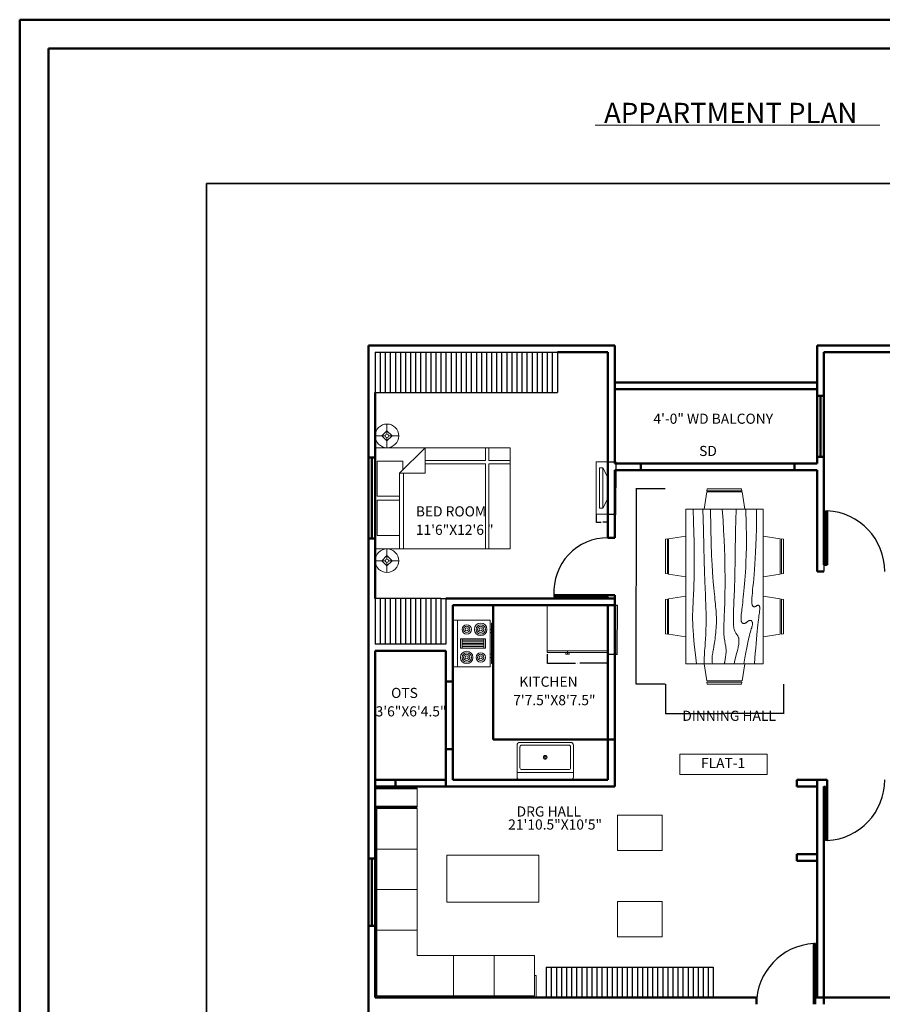
# Model space of a CAD drawing. Units: inches. Extents: x 1493 to 2377, y 814 to 2191.
# Tile 3 of 4: x 1493 to 2004, y 1607 to 2191. Entities that reach past the tile are written whole.
import ezdxf

# ---------------------------------------------------------------- set-up
doc = ezdxf.new("R2010")
doc.units = ezdxf.units.IN
for name, color, linetype, lineweight in [('A-ANNO-DIMS', 2, 'Continuous', 18), ('A-ANNO-SYMB', 2, 'Continuous', 18), ('A-ANNO-TEXT', 3, 'Continuous', 18), ('A-ANNO-TTLB', 7, 'Continuous', 35), ('A-AREA-IDEN', 7, 'Continuous', 18), ('A-DOOR', 4, 'Continuous', 25), ('A-EQPM', 9, 'Continuous', 18), ('A-FLOR-FIXT', 8, 'Continuous', 18), ('A-FURN', 8, 'Continuous', 18), ('A-GLAZ', 4, 'Continuous', 25), ('A-WALL', 7, 'Continuous', 50)]:
    doc.layers.add(name, color=color, linetype=linetype, lineweight=lineweight)
doc.styles.get("Standard").update_dxf_attribs({"font": 'arial.ttf'})
doc.dimstyles.get("Standard").update_dxf_attribs({"dimtxt": 0.18, "dimasz": 0.18, "dimexe": 0.18, "dimexo": 0.0625, "dimgap": 0.09, "dimtad": 0, "dimtih": 1, "dimtoh": 1, "dimdec": 4, "dimzin": 0, "dimdsep": 46, "dimtxsty": 'Standard', "dimcen": 0.09, "dimadec": 0, "dimazin": 0, "dimtfac": 1, "dimtdec": 4, "dimtofl": 0, "dimtmove": 0, "dimatfit": 3, "dimfxl": 1, "dimtolj": 1, "dimtzin": 0, "dimarcsym": 0})

# ---------------------------------------------------------------- blocks, each defined once
blk = doc.blocks.new('Lamp - Table')
for p, q in [((0, 7), (0, 1)), ((-1, 0), (-7, 0)), ((0, 3), (-3, 0)), ((-3, 0), (0, -3)), ((3, 0), (0, 3)), ((0, -3), (3, 0)), ((1, 0), (7, 0)), ((0, -1), (0, -7))]:
    blk.add_line(p, q)
for radius in [7, 1]:
    blk.add_circle((0, 0), radius)
blk = doc.blocks.new('Range-Oven - 30 in top')
for p, q in [((0, -3), (30, -3)), ((12, -6), (18, -6)), ((13, -20), (13, -6)), ((14, -6), (14, -20)), ((15, -20), (15, -6)), ((16, -6), (16, -20)), ((17, -20), (17, -6)), ((6, -24), (6, -25)), ((8, -25), (8, -24)), ((18, -20), (12, -20)), ((22, -25), (22, -24)), ((24, -24), (24, -25))]:
    blk.add_line(p, q)
for points in [[(0, -24), (0, 0), (30, 0), (30, -24)], [(12, -21), (12, -5), (18, -5), (18, -21)], [(2, -26), (2, -25), (28, -25), (28, -26)]]:
    blk.add_lwpolyline(points, close=True)
for centre, radius in [((6, -9), 4), ((6, -9), 3), ((24, -9), 3), ((6, -9), 2), ((6, -9), 1), ((24, -9), 2), ((24, -9), 1), ((6, -18), 3), ((6, -18), 2), ((6, -18), 1), ((24, -18), 4), ((24, -18), 3), ((24, -18), 2), ((24, -18), 1)]:
    blk.add_circle(centre, radius)
blk = doc.blocks.new('Refrigerator-2 door - 36 in top')
for p, q in [((0, -26.999999), (36, -26.999999)), ((11, -27.999999), (11, -28.999999)), ((11, -28.999999), (13, -28.999999)), ((12, -26.999999), (12, -28.999999)), ((13, -28.999999), (13, -27.999999))]:
    blk.add_line(p, q)
blk.add_lwpolyline([(0, -27.999999), (0, 0), (36, 0), (36, -27.999999)], close=True)
blk = doc.blocks.new('Bed - Queen')
for p, q in [((0, -80), (0, 0)), ((0, 0), (60, 0)), ((60, 0), (60, -80)), ((8, -1.2), (28.8, -1.2)), ((8, -14.4), (8, -1.2)), ((28.8, -1.2), (28.8, -14.4)), ((31.2, -1.2), (52, -1.2)), ((31.2, -14.4), (31.2, -1.2)), ((52, -1.2), (52, -16.4)), ((0, -14.4), (44.8, -14.4)), ((44.8, -16.8), (0, -16.8)), ((60, -29.6), (44.8, -14.4)), ((44.8, -14.4), (44.8, -29.6)), ((52, -16.4), (46.8, -16.4)), ((44.8, -29.6), (60, -29.6)), ((50.4, -29.6), (50.4, -65.35)), ((52.4, -29.6), (52.4, -65.35)), ((50.4, -65.35), (0, -65.35)), ((50.4, -67.35), (0, -67.35)), ((50.4, -67.35), (50.4, -80)), ((60, -65.35), (52.4, -65.35)), ((60, -67.35), (52.4, -67.35)), ((52.4, -67.35), (52.4, -80)), ((60, -80), (0, -80))]:
    blk.add_line(p, q)
blk = doc.blocks.new('Sink-single - 30 in top')
blk.add_line((-15, -3.999996), (15, -3.999996))
for points in [[(-13.5, 0), (13.5, 0)], [(-15, -18.499996), (-15, -1.5)], [(15, -1.5), (15, -18.499996)], [(-13.5, -17.499996), (-13.5, -6.499996)], [(-12.5, -5.499996), (12.5, -5.499996)], [(13.5, -6.499996), (13.5, -17.499996)], [(13.5, -19.999996), (-13.5, -19.999996)], [(12.5, -18.499996), (-12.5, -18.499996)]]:
    blk.add_lwpolyline(points)
for radius in [1, 0.5]:
    blk.add_circle((0, -11.999996), radius)
for centre, radius, start, end in [((-13.5, -1.5), 1.5, 90, 180), ((13.5, -1.5), 1.5, 0, 90), ((-12.5, -6.499996), 1, 90, 180), ((12.5, -6.499996), 1, 0, 90), ((-13.5, -18.499996), 1.5, 180, 270), ((-12.5, -17.499996), 1, 180, 270), ((12.5, -17.499996), 1, 270, 0), ((13.5, -18.499996), 1.5, 270, 0)]:
    blk.add_arc(centre, radius, start, end)
blk = doc.blocks.new('Dining Set - 36 x 72 in.')
for p, q in [((-22, 27.5), (-22.1562, 26.50042)), ((-22, 27.5), (-6, 27.5)), ((-5.8437, 26.49966), (-6, 27.5)), ((6, 27.5), (5.8438, 26.50042)), ((6, 27.5), (22, 27.5)), ((22.1563, 26.49966), (22, 27.5)), ((-22.2343, 26.00059), (-23.4847, 17.99762)), ((-22.2304, 26), (-5.7608, 26)), ((-5.8416, 26.5), (-22.1534, 26.5)), ((-4.5152, 17.99762), (-5.7655, 25.99926)), ((5.7657, 26.00059), (4.5153, 17.99762)), ((5.7696, 26), (22.2392, 26)), ((22.1584, 26.5), (5.8466, 26.5)), ((23.4848, 17.99762), (22.2345, 25.99926)), ((36, 18), (-36, 18)), ((-36, 18), (-36, -18)), ((36, -18), (36, 18)), ((-44.0006, 8.23428), (-35.9976, 9.48474)), ((44.0006, 8.23428), (35.9976, 9.48474)), ((-45.5, 8), (-44.5004, 8.15617)), ((-45.5, 8), (-45.5, -8)), ((-44.5, -8.15843), (-44.5, 8.15338)), ((-44, 8.23041), (-44, -8.23915)), ((44, 8.23041), (44, -8.23915)), ((44.5, -8.15843), (44.5, 8.15338)), ((45.5, 8), (44.5005, 8.15617)), ((45.5, 8), (45.5, -8)), ((-44.4997, -8.15631), (-45.5, -8)), ((-35.9976, -9.48476), (-43.9993, -8.2345)), ((35.9976, -9.48476), (43.9993, -8.2345)), ((44.4997, -8.15631), (45.5, -8)), ((-36, -18), (36, -18)), ((-22.2343, -26.0006), (-23.4847, -17.99762)), ((-4.5152, -17.99762), (-5.7655, -25.99928)), ((5.7657, -26.0006), (4.5153, -17.99762)), ((23.4848, -17.99762), (22.2345, -25.99928)), ((-22.2304, -26), (-5.7608, -26)), ((-22, -27.5), (-22.1562, -26.50044)), ((-5.8416, -26.5), (-22.1534, -26.5)), ((-5.8437, -26.49967), (-6, -27.5)), ((5.7696, -26), (22.2392, -26)), ((6, -27.5), (5.8438, -26.50044)), ((22.1584, -26.5), (5.8466, -26.5)), ((22.1563, -26.49967), (22, -27.5)), ((-22, -27.5), (-6, -27.5)), ((6, -27.5), (22, -27.5))]:
    blk.add_line(p, q)
for points in [[(-36, 15), (-31.1772, 14.97754), (-26.8079, 14.91406), (-22.8538, 14.81543), (-19.276, 14.6875), (-16.0362, 14.53613), (-13.0957, 14.36718), (-10.4159, 14.18652), (-7.9583, 14), (-5.6904, 13.81315), (-3.6035, 13.63021), (-1.6954, 13.45508), (0.0365, 13.29166), (1.5945, 13.14388), (2.9811, 13.01562), (4.1988, 12.9108), (5.25, 12.83333), (6.1393, 12.78613), (6.8802, 12.76823), (7.4883, 12.77767), (7.9792, 12.8125), (8.3685, 12.87077), (8.6719, 12.95052), (8.9049, 13.0498), (9.0833, 13.16666), (9.2205, 13.29899), (9.3216, 13.44401), (9.3895, 13.59879), (9.4271, 13.76041), (9.4373, 13.92594), (9.4232, 14.09245), (9.3875, 14.257), (9.3333, 14.41666), (9.2638, 14.56917), (9.1836, 14.71484), (9.0975, 14.85465), (9.0104, 14.98958), (8.9272, 15.1206), (8.8529, 15.2487), (8.7922, 15.37483), (8.75, 15.5), (8.7305, 15.62467), (8.7344, 15.74739), (8.7617, 15.86621), (8.8125, 15.97916), (8.8867, 16.08431), (8.9844, 16.17968), (9.1055, 16.26334), (9.25, 16.33333), (9.4189, 16.38802), (9.6172, 16.42708), (9.8506, 16.45052), (10.125, 16.45833), (10.4463, 16.45052), (10.8203, 16.42708), (11.2529, 16.38802), (11.75, 16.33333), (12.3184, 16.26318), (12.9694, 16.17838), (13.7151, 16.07991), (14.5677, 15.96875), (15.5395, 15.84586), (16.6426, 15.71224), (17.8893, 15.56884), (19.2917, 15.41666), (20.859, 15.25667), (22.5879, 15.08984), (24.4721, 14.91715), (26.5052, 14.73958), (28.6809, 14.5581), (30.9929, 14.3737), (33.4347, 14.18733), (36, 14)], [(-36, 10), (-28.9766, 10.14274), (-23.1725, 10.20442), (-18.4241, 10.19775), (-14.5677, 10.13541), (-11.4399, 10.03011), (-8.877, 9.89453), (-6.7154, 9.74137), (-4.7917, 9.58333), (-2.9698, 9.43082), (-1.2246, 9.28515), (0.4415, 9.14534), (2.026, 9.01041), (3.5266, 8.87939), (4.9408, 8.7513), (6.266, 8.62516), (7.5, 8.5), (8.6411, 8.37549), (9.6914, 8.2539), (10.6538, 8.13818), (11.5312, 8.03125), (12.3267, 7.93603), (13.043, 7.85547), (13.6831, 7.79248), (14.25, 7.75), (14.7471, 7.7303), (15.1797, 7.73307), (15.5537, 7.75732), (15.875, 7.80208), (16.1494, 7.86637), (16.3828, 7.94922), (16.5811, 8.04964), (16.75, 8.16666), (16.8944, 8.29915), (17.0143, 8.44531), (17.1089, 8.60319), (17.1771, 8.77083), (17.218, 8.94629), (17.2305, 9.1276), (17.2137, 9.31282), (17.1667, 9.5), (17.0895, 9.6875), (16.987, 9.875), (16.8649, 10.0625), (16.7292, 10.25), (16.5856, 10.4375), (16.4401, 10.625), (16.2985, 10.8125), (16.1667, 11), (16.05, 11.18733), (15.9518, 11.3737), (15.8752, 11.5581), (15.8229, 11.73958), (15.798, 11.91715), (15.8034, 12.08984), (15.842, 12.25667), (15.9167, 12.41666), (16.0295, 12.56836), (16.1784, 12.70833), (16.3605, 12.83268), (16.5729, 12.9375), (16.8127, 13.01888), (17.0768, 13.07291), (17.3625, 13.0957), (17.6667, 13.08333), (17.9894, 13.03312), (18.3418, 12.94726), (18.7382, 12.82918), (19.1927, 12.68229), (19.7195, 12.51001), (20.3327, 12.31575), (21.0465, 12.10294), (21.875, 11.875), (22.8357, 11.63354), (23.959, 11.37304), (25.2786, 11.08618), (26.8282, 10.76562), (28.6414, 10.40405), (30.752, 9.99414), (33.1936, 9.52856), (36, 9)], [(-36, 5.5), (-30.7157, 5.3348), (-26.069, 5.20963), (-21.9946, 5.11767), (-18.4271, 5.05208), (-15.3009, 5.00602), (-12.5508, 4.97265), (-10.1112, 4.94515), (-7.9167, 4.91666), (-5.909, 4.88167), (-4.0586, 4.83984), (-2.3429, 4.79215), (-0.7396, 4.73958), (0.7739, 4.6831), (2.22, 4.6237), (3.6213, 4.56233), (5, 4.5), (6.373, 4.43782), (7.7344, 4.3776), (9.0723, 4.32129), (10.375, 4.27083), (11.6309, 4.22819), (12.8281, 4.19531), (13.9551, 4.17415), (15, 4.16666), (15.954, 4.17448), (16.819, 4.19791), (17.6001, 4.23698), (18.3021, 4.29166), (18.9299, 4.36198), (19.4883, 4.44791), (19.9823, 4.54948), (20.4167, 4.66666), (20.7969, 4.79899), (21.1302, 4.94401), (21.4245, 5.09879), (21.6875, 5.26041), (21.9271, 5.42594), (22.1511, 5.59245), (22.3672, 5.757), (22.5834, 5.91666), (22.8065, 6.06868), (23.0404, 6.21093), (23.2879, 6.34147), (23.5521, 6.45833), (23.8358, 6.55957), (24.142, 6.64323), (24.4735, 6.70735), (24.8334, 6.75), (25.2235, 6.76969), (25.642, 6.76692), (26.0858, 6.74267), (26.5521, 6.69791), (27.0379, 6.63362), (27.5404, 6.55078), (28.0565, 6.45036), (28.5834, 6.33333), (29.1242, 6.19987), (29.7071, 6.04687), (30.3661, 5.87044), (31.1354, 5.66666), (32.0493, 5.43164), (33.142, 5.16146), (34.4475, 4.85221), (36, 4.5)], [(-36, -1), (-30.7915, -0.6591), (-26.0195, -0.38216), (-21.6519, -0.16284), (-17.6563, 0.00521), (-14.0005, 0.12833), (-10.6523, 0.21289), (-7.5796, 0.26522), (-4.75, 0.29166), (-2.134, 0.29793), (0.2878, 0.28711), (2.5317, 0.26163), (4.6146, 0.22396), (6.5529, 0.17651), (8.3633, 0.12174), (10.0623, 0.06209), (11.6667, 0), (13.1899, -0.06201), (14.6341, -0.1211), (15.9982, -0.17432), (17.2813, -0.21875), (18.4823, -0.25147), (19.6003, -0.26953), (20.6343, -0.27002), (21.5834, -0.25), (22.4481, -0.20768), (23.2357, -0.14584), (23.9549, -0.06836), (24.6146, 0.02083), (25.2235, 0.11784), (25.7904, 0.21875), (26.3241, 0.31966), (26.8334, 0.41666), (27.3265, 0.50618), (27.8099, 0.58593), (28.2894, 0.65397), (28.7709, 0.70833), (29.2601, 0.74707), (29.763, 0.76823), (30.2855, 0.76985), (30.8334, 0.75), (31.4088, 0.70784), (31.9994, 0.64713), (32.589, 0.57275), (33.1615, 0.48958), (33.7008, 0.4025), (34.1908, 0.3164), (34.6153, 0.23616), (34.9584, 0.16666), (35.2099, 0.11165), (35.3848, 0.07031), (35.504, 0.04069), (35.5886, 0.02083), (35.6594, 0.00879), (35.7377, 0.0026), (35.8442, 0.00032), (36, 0)], [(-36, -6.5), (-27.1843, -6.31267), (-20.084, -6.1263), (-14.469, -5.9419), (-10.1094, -5.76042), (-6.7752, -5.58285), (-4.2363, -5.41016), (-2.2629, -5.24333), (-0.625, -5.08334), (0.8708, -4.93099), (2.2715, -4.78646), (3.5872, -4.64974), (4.8281, -4.52084), (6.0046, -4.39974), (7.127, -4.28646), (8.2053, -4.18099), (9.25, -4.08334), (10.2705, -3.99382), (11.2734, -3.91407), (12.2647, -3.84603), (13.25, -3.79167), (14.2354, -3.75293), (15.2266, -3.73177), (16.2295, -3.73015), (17.25, -3.75), (18.2912, -3.79248), (19.3451, -3.85547), (20.4009, -3.93604), (21.4479, -4.03125), (22.4754, -4.13819), (23.4727, -4.25391), (24.4289, -4.37549), (25.3334, -4.5), (26.1785, -4.62492), (26.9694, -4.74935), (27.7145, -4.87281), (28.4219, -4.99479), (29.1, -5.11483), (29.7572, -5.23242), (30.4016, -5.34709), (31.0417, -5.45834), (31.6837, -5.56437), (32.3262, -5.65821), (32.9658, -5.73153), (33.599, -5.77604), (34.2224, -5.78345), (34.8327, -5.74545), (35.4264, -5.65373), (36, -5.5)], [(-36, -10), (-26.4022, -9.81299), (-18.4675, -9.62891), (-11.9839, -9.45069), (-6.7396, -9.28125), (-2.5226, -9.12354), (0.8789, -8.98047), (3.6769, -8.85498), (6.0833, -8.75), (8.2767, -8.66765), (10.3021, -8.60677), (12.1712, -8.56543), (13.8958, -8.54167), (15.4876, -8.53353), (16.9583, -8.53907), (18.3197, -8.55632), (19.5834, -8.58334), (20.7616, -8.61841), (21.8685, -8.66081), (22.9188, -8.71004), (23.9271, -8.76563), (24.9081, -8.82707), (25.8763, -8.89388), (26.8465, -8.96558), (27.8334, -9.04167), (28.8474, -9.12118), (29.8828, -9.20117), (30.93, -9.27824), (31.9792, -9.34896), (33.0205, -9.40991), (34.0443, -9.45768), (35.0407, -9.48885), (36, -9.5)], [(-36, -14.5), (-30.0881, -14.33513), (-25.0332, -14.21224), (-20.7312, -14.12647), (-17.0781, -14.07292), (-13.97, -14.04671), (-11.3027, -14.04297), (-8.9724, -14.05681), (-6.875, -14.08334), (-4.9224, -14.11833), (-3.0905, -14.16016), (-1.3709, -14.20785), (0.2448, -14.26042), (1.7647, -14.3169), (3.1973, -14.3763), (4.5507, -14.43767), (5.8333, -14.5), (7.0554, -14.5621), (8.235, -14.62175), (9.3922, -14.67652), (10.5469, -14.72396), (11.7192, -14.76164), (12.929, -14.78711), (14.1965, -14.79794), (15.5417, -14.79167), (16.9933, -14.76424), (18.6152, -14.70508), (20.4804, -14.60197), (22.6615, -14.44271), (25.2312, -14.21509), (28.2624, -13.9069), (31.8277, -13.50594), (36, -13)]]:
    blk.add_lwpolyline(points)
blk = doc.blocks.new('AC-SPLIT-UNIT')
for p, q in [((-2, 27.5), (-2, -3.65)), ((-2, 27.5), (5, 27.5)), ((0, 24), (2, 24)), ((0, 24), (0, 0)), ((2, 24), (2, 0)), ((2, 24), (5, 18.22)), ((2, 0), (5, 5.78)), ((-2, -3.65), (5, -3.65)), ((0, 0), (2, 0))]:
    blk.add_line(p, q)
blk = doc.blocks.new('*D24')
at = {"layer": 'A-ANNO-DIMS', "color": 0, "lineweight": -2, "transparency": 16777216}
for p, q in [((1841.9, 1928.89), (1846.69, 1928.89)), ((1846.51, 1928.71), (1846.51, 1913.5)), ((1846.51, 1897.92), (1846.51, 1913.13)), ((1841.9, 1897.74), (1846.69, 1897.74))]:
    blk.add_line(p, q, dxfattribs=at)
at = {"layer": 'A-ANNO-DIMS', "color": 0, "transparency": 16777216}
for points in [[(1846.48, 1928.71), (1846.54, 1928.71), (1846.51, 1928.89)], [(1846.48, 1897.92), (1846.54, 1897.92), (1846.51, 1897.74)]]:
    blk.add_solid(points, dxfattribs=at)
at = {"layer": 'Defpoints', "color": 0, "transparency": 16777216}
for p in [(1841.83, 1928.89), (1846.51, 1928.89), (1841.83, 1897.74)]:
    blk.add_point(p, dxfattribs=at)
at = {"layer": 'A-ANNO-DIMS', "color": 0, "transparency": 16777216, "insert": (1846.51, 1913.32), "char_height": 0.18, "attachment_point": 5}
blk.add_mtext('\\A1;AC SPLIT UNIT 31 TYP.', dxfattribs=at)
blk = doc.blocks.new('*D25')
at = {"layer": 'A-ANNO-DIMS', "color": 0, "lineweight": -2, "transparency": 16777216}
for p, q in [((1834.83, 1897.68), (1834.83, 1892.89)), ((1841.83, 1897.68), (1841.83, 1892.89)), ((1835.01, 1893.07), (1837.88, 1893.07)), ((1841.65, 1893.07), (1838.79, 1893.07))]:
    blk.add_line(p, q, dxfattribs=at)
at = {"layer": 'A-ANNO-DIMS', "color": 0, "transparency": 16777216}
for points in [[(1835.01, 1893.1), (1835.01, 1893.04), (1834.83, 1893.07)], [(1841.65, 1893.1), (1841.65, 1893.04), (1841.83, 1893.07)]]:
    blk.add_solid(points, dxfattribs=at)
at = {"layer": 'Defpoints', "color": 0, "transparency": 16777216}
for p in [(1834.83, 1897.74), (1841.83, 1897.74), (1841.83, 1893.07)]:
    blk.add_point(p, dxfattribs=at)
at = {"layer": 'A-ANNO-DIMS', "color": 0, "transparency": 16777216, "insert": (1838.33, 1893.07), "char_height": 0.18, "attachment_point": 5}
blk.add_mtext('\\A1;7 TYP.', dxfattribs=at)
blk = doc.blocks.new('*D30')
at = {"layer": 'A-ANNO-DIMS', "color": 0, "lineweight": -2, "transparency": 16777216}
for p, q in [((1875.78, 1912.92), (1858.28, 1912.92)), ((1858.46, 1912.74), (1858.46, 1855.18)), ((1858.46, 1797.25), (1858.46, 1854.81)), ((1875.78, 1797.07), (1858.28, 1797.07))]:
    blk.add_line(p, q, dxfattribs=at)
at = {"layer": 'A-ANNO-DIMS', "color": 0, "transparency": 16777216}
for points in [[(1858.43, 1912.74), (1858.49, 1912.74), (1858.46, 1912.92)], [(1858.43, 1797.25), (1858.49, 1797.25), (1858.46, 1797.07)]]:
    blk.add_solid(points, dxfattribs=at)
at = {"layer": 'Defpoints', "color": 0, "transparency": 16777216}
for p in [(1875.84, 1912.92), (1858.46, 1797.07), (1875.84, 1797.07)]:
    blk.add_point(p, dxfattribs=at)
at = {"layer": 'A-ANNO-DIMS', "color": 0, "transparency": 16777216, "insert": (1858.46, 1854.99), "char_height": 0.18, "attachment_point": 5}
blk.add_mtext('\\A1;DINING SET 116', dxfattribs=at)
blk = doc.blocks.new('*D31')
at = {"layer": 'A-ANNO-DIMS', "color": 0, "lineweight": -2, "transparency": 16777216}
for p, q in [((1875.84, 1797), (1875.84, 1779.51)), ((1945.87, 1797), (1945.87, 1779.51)), ((1876.02, 1779.69), (1910.64, 1779.69)), ((1945.69, 1779.69), (1911.07, 1779.69))]:
    blk.add_line(p, q, dxfattribs=at)
at = {"layer": 'A-ANNO-DIMS', "color": 0, "transparency": 16777216}
for points in [[(1876.02, 1779.72), (1876.02, 1779.66), (1875.84, 1779.69)], [(1945.69, 1779.72), (1945.69, 1779.66), (1945.87, 1779.69)]]:
    blk.add_solid(points, dxfattribs=at)
at = {"layer": 'Defpoints', "color": 0, "transparency": 16777216}
for p in [(1875.84, 1797.07), (1945.87, 1797.07), (1945.87, 1779.69)]:
    blk.add_point(p, dxfattribs=at)
at = {"layer": 'A-ANNO-DIMS', "color": 0, "transparency": 16777216, "insert": (1910.85, 1779.69), "char_height": 0.18, "attachment_point": 5}
blk.add_mtext('\\A1;70', dxfattribs=at)
blk = doc.blocks.new('*D34')
at = {"layer": 'A-ANNO-DIMS', "color": 0, "lineweight": -2, "transparency": 16777216}
for p, q in [((1805.83, 1814.8), (1805.83, 1809.29)), ((1841.83, 1814.8), (1841.83, 1809.29)), ((1806.01, 1809.47), (1822.58, 1809.47)), ((1841.65, 1809.47), (1825.08, 1809.47))]:
    blk.add_line(p, q, dxfattribs=at)
at = {"layer": 'A-ANNO-DIMS', "color": 0, "transparency": 16777216}
for points in [[(1806.01, 1809.5), (1806.01, 1809.44), (1805.83, 1809.47)], [(1841.65, 1809.5), (1841.65, 1809.44), (1841.83, 1809.47)]]:
    blk.add_solid(points, dxfattribs=at)
at = {"layer": 'Defpoints', "color": 0, "transparency": 16777216}
for p in [(1805.83, 1814.87), (1841.83, 1814.87), (1841.83, 1809.47)]:
    blk.add_point(p, dxfattribs=at)
at = {"layer": 'A-ANNO-DIMS', "color": 0, "transparency": 16777216, "insert": (1823.83, 1809.47), "char_height": 0.18, "attachment_point": 5}
blk.add_mtext('\\A1;REFRIGERATOR 36', dxfattribs=at)
blk = doc.blocks.new('*D35')
at = {"layer": 'A-ANNO-DIMS', "color": 0, "lineweight": -2, "transparency": 16777216}
for p, q in [((1841.9, 1843.87), (1847.41, 1843.87)), ((1847.23, 1843.69), (1847.23, 1829.55)), ((1847.23, 1815.05), (1847.23, 1829.19)), ((1841.9, 1814.87), (1847.41, 1814.87))]:
    blk.add_line(p, q, dxfattribs=at)
at = {"layer": 'A-ANNO-DIMS', "color": 0, "transparency": 16777216}
for points in [[(1847.2, 1843.69), (1847.26, 1843.69), (1847.23, 1843.87)], [(1847.2, 1815.05), (1847.26, 1815.05), (1847.23, 1814.87)]]:
    blk.add_solid(points, dxfattribs=at)
at = {"layer": 'Defpoints', "color": 0, "transparency": 16777216}
for p in [(1841.83, 1843.87), (1847.23, 1843.87), (1841.83, 1814.87)]:
    blk.add_point(p, dxfattribs=at)
at = {"layer": 'A-ANNO-DIMS', "color": 0, "transparency": 16777216, "insert": (1847.23, 1829.37), "char_height": 0.18, "attachment_point": 5}
blk.add_mtext('\\A1;29', dxfattribs=at)

msp = doc.modelspace()

# ---------------------------------------------------------------- linework, layer by layer
at = {"layer": 'A-ANNO-SYMB'}
msp.add_lwpolyline([(1884.39, 1755.7), (1936.09, 1755.7), (1936.09, 1743.61), (1884.39, 1743.61)], close=True, dxfattribs=at)
at = {"layer": 'A-ANNO-TEXT'}
msp.add_line((1834.32, 2128.42), (2002.99, 2128.42), dxfattribs=at)
at = {"layer": 'A-ANNO-TTLB'}
for q in [(1603.83, 914.87), (2271.83, 2093.87)]:
    msp.add_line((1603.83, 2093.87), q, dxfattribs=at)
at = {"layer": 'A-DOOR'}
for p, q in [((1970.83, 1899.87), (1971.83, 1899.87)), ((1970.83, 1899.87), (1970.83, 1867.87)), ((1969.83, 1867.87), (1969.83, 1863.87)), ((1809.83, 1849.87), (1809.83, 1848.87)), ((1970.83, 1736.37), (1969.83, 1736.37)), ((1970.83, 1736.37), (1970.83, 1704.37)), ((1971.83, 1704.37), (1970.83, 1704.37)), ((1964.83, 1643.37), (1963.83, 1643.37)), ((1964.83, 1643.37), (1964.83, 1607.37))]:
    msp.add_line(p, q, dxfattribs=at)
for centre, radius, start, end in [((1969.77, 1863.87), 36.06, 0, 86.72685), ((1841.83, 1851.81), 32.06, 90, 183.47141), ((1969.77, 1740.37), 36.06, 273.27315, 360), ((1965.89, 1607.37), 36.06, 93.27315, 180)]:
    msp.add_arc(centre, radius, start, end, dxfattribs=at)
at = {"layer": 'A-FURN'}
for p, q in [((1728.83, 1724.37), (1728.83, 1735.37)), ((1704.83, 1723.37), (1704.83, 1612.37)), ((1728.83, 1723.37), (1704.83, 1723.37)), ((1709.83, 1724.37), (1709.83, 1723.37)), ((1728.83, 1723.37), (1728.83, 1636.37)), ((1728.83, 1699.37), (1704.83, 1699.37)), ((1728.83, 1675.37), (1704.83, 1675.37)), ((1728.83, 1651.37), (1704.83, 1651.37)), ((1798.36, 1636.37), (1728.83, 1636.37)), ((1750.36, 1636.37), (1750.36, 1612.37)), ((1774.36, 1636.37), (1774.36, 1612.37)), ((1798.36, 1636.37), (1798.36, 1612.37)), ((1799.36, 1624.37), (1798.36, 1624.37)), ((1799.36, 1624.37), (1799.36, 1611.37)), ((1798.36, 1612.37), (1704.83, 1612.37))]:
    msp.add_line(p, q, dxfattribs=at)
for points in [[(1847.43, 1719.55), (1873.89, 1719.55), (1873.89, 1698.59), (1847.43, 1698.59)], [(1746.4, 1695.69), (1800.95, 1695.69), (1800.95, 1667.95), (1746.4, 1667.95)], [(1847.43, 1668.28), (1873.89, 1668.28), (1873.89, 1647.31), (1847.43, 1647.31)]]:
    msp.add_lwpolyline(points, close=True, dxfattribs=at)
at = {"layer": 'A-GLAZ'}
for p, q in [((1703.83, 1993.87), (1808.83, 1993.87)), ((1703.83, 1993.87), (1703.83, 1969.87)), ((1706.83, 1993.87), (1706.83, 1969.87)), ((1709.83, 1993.87), (1709.83, 1969.87)), ((1712.83, 1993.87), (1712.83, 1969.87)), ((1715.83, 1993.87), (1715.83, 1969.87)), ((1718.83, 1993.87), (1718.83, 1969.87)), ((1721.83, 1993.87), (1721.83, 1969.87)), ((1724.83, 1993.87), (1724.83, 1969.87)), ((1727.83, 1993.87), (1727.83, 1969.87)), ((1730.83, 1993.87), (1730.83, 1969.87)), ((1733.83, 1993.87), (1733.83, 1969.87)), ((1736.83, 1993.87), (1736.83, 1969.87)), ((1739.83, 1993.87), (1739.83, 1969.87)), ((1742.83, 1993.87), (1742.83, 1969.87)), ((1745.83, 1993.87), (1745.83, 1969.87)), ((1748.83, 1993.87), (1748.83, 1969.87)), ((1751.83, 1993.87), (1751.83, 1969.87)), ((1754.83, 1993.87), (1754.83, 1969.87)), ((1757.83, 1993.87), (1757.83, 1969.87)), ((1760.83, 1993.87), (1760.83, 1969.87)), ((1763.83, 1993.87), (1763.83, 1969.87)), ((1766.83, 1993.87), (1766.83, 1969.87)), ((1769.83, 1993.87), (1769.83, 1969.87)), ((1772.83, 1993.87), (1772.83, 1969.87)), ((1775.83, 1993.87), (1775.83, 1969.87)), ((1778.83, 1993.87), (1778.83, 1969.87)), ((1781.83, 1993.87), (1781.83, 1969.87)), ((1784.83, 1993.87), (1784.83, 1969.87)), ((1787.83, 1993.87), (1787.83, 1969.87)), ((1790.83, 1993.87), (1790.83, 1969.87)), ((1793.83, 1993.87), (1793.83, 1969.87)), ((1796.83, 1993.87), (1796.83, 1969.87)), ((1799.83, 1993.87), (1799.83, 1969.87)), ((1802.83, 1993.87), (1802.83, 1969.87)), ((1805.83, 1993.87), (1805.83, 1969.87)), ((1808.83, 1993.87), (1808.83, 1969.87)), ((1808.83, 1993.87), (1811.83, 1993.87)), ((1811.83, 1993.87), (1811.83, 1969.87)), ((1703.83, 1969.87), (1811.83, 1969.87)), ((1742.83, 1847.87), (1703.83, 1847.87)), ((1703.83, 1847.87), (1703.83, 1820.87)), ((1706.83, 1847.87), (1706.83, 1820.87)), ((1709.83, 1847.87), (1709.83, 1820.87)), ((1712.83, 1847.87), (1712.83, 1820.87)), ((1715.83, 1847.87), (1715.83, 1820.87)), ((1718.83, 1847.87), (1718.83, 1820.87)), ((1721.83, 1847.87), (1721.83, 1820.87)), ((1724.83, 1847.87), (1724.83, 1820.87)), ((1727.83, 1847.87), (1727.83, 1820.87)), ((1730.83, 1847.87), (1730.83, 1820.87)), ((1733.83, 1847.87), (1733.83, 1820.87)), ((1736.83, 1847.87), (1736.83, 1820.87)), ((1739.83, 1847.87), (1739.83, 1820.87)), ((1742.83, 1847.87), (1742.83, 1820.87)), ((1742.83, 1847.87), (1745.83, 1847.87)), ((1745.83, 1847.87), (1745.83, 1820.87)), ((1745.83, 1820.87), (1703.83, 1820.87)), ((1805.27, 1629.37), (1904.27, 1629.37)), ((1805.27, 1629.37), (1805.27, 1611.37)), ((1808.27, 1629.37), (1808.27, 1611.37)), ((1811.27, 1629.37), (1811.27, 1611.37)), ((1814.27, 1629.37), (1814.27, 1611.37)), ((1817.27, 1629.37), (1817.27, 1611.37)), ((1820.27, 1629.37), (1820.27, 1611.37)), ((1823.27, 1629.37), (1823.27, 1611.37)), ((1826.27, 1629.37), (1826.27, 1611.37)), ((1829.27, 1629.37), (1829.27, 1611.37)), ((1832.27, 1629.37), (1832.27, 1611.37)), ((1835.27, 1629.37), (1835.27, 1611.37)), ((1838.27, 1629.37), (1838.27, 1611.37)), ((1841.27, 1629.37), (1841.27, 1611.37)), ((1844.27, 1629.37), (1844.27, 1611.37)), ((1847.27, 1629.37), (1847.27, 1611.37)), ((1850.27, 1629.37), (1850.27, 1611.37)), ((1853.27, 1629.37), (1853.27, 1611.37)), ((1856.27, 1629.37), (1856.27, 1611.37)), ((1859.27, 1629.37), (1859.27, 1611.37)), ((1862.27, 1629.37), (1862.27, 1611.37)), ((1865.27, 1629.37), (1865.27, 1611.37)), ((1868.27, 1629.37), (1868.27, 1611.37)), ((1871.27, 1629.37), (1871.27, 1611.37)), ((1874.27, 1629.37), (1874.27, 1611.37)), ((1877.27, 1629.37), (1877.27, 1611.37)), ((1880.27, 1629.37), (1880.27, 1611.37)), ((1883.27, 1629.37), (1883.27, 1611.37)), ((1886.27, 1629.37), (1886.27, 1611.37)), ((1889.27, 1629.37), (1889.27, 1611.37)), ((1892.27, 1629.37), (1892.27, 1611.37)), ((1895.27, 1629.37), (1895.27, 1611.37)), ((1898.27, 1629.37), (1898.27, 1611.37)), ((1901.27, 1629.37), (1901.27, 1611.37)), ((1904.27, 1629.37), (1904.27, 1611.37))]:
    msp.add_line(p, q, dxfattribs=at)
at = {"layer": 'A-WALL'}
for p, q in [((1699.83, 1997.87), (1845.83, 1997.87)), ((1699.83, 1997.87), (1699.83, 1010.87)), ((1845.83, 1997.87), (1845.83, 1927.87)), ((1965.83, 1997.87), (1965.83, 1927.87)), ((1965.83, 1997.87), (2151.83, 1997.87)), ((1965.83, 1997.87), (1965.83, 1927.87)), ((1811.83, 1993.87), (1841.83, 1993.87)), ((1841.83, 1993.87), (1841.83, 1883.87)), ((1969.83, 1993.87), (1969.83, 1867.87)), ((1969.83, 1993.87), (1969.83, 1867.87)), ((1969.83, 1993.87), (2125.83, 1993.87)), ((1845.83, 1975.87), (1965.83, 1975.87)), ((1703.83, 1969.87), (1703.83, 1847.87)), ((1845.83, 1971.87), (1965.83, 1971.87)), ((1965.83, 1967.87), (1969.83, 1967.87)), ((1967.83, 1967.87), (1967.83, 1931.87)), ((1965.83, 1931.87), (1969.83, 1931.87)), ((1703.83, 1931.37), (1699.83, 1931.37)), ((1701.83, 1931.37), (1701.83, 1883.37)), ((1845.83, 1927.87), (1965.83, 1927.87)), ((1861.27, 1927.87), (1861.27, 1923.87)), ((1952.36, 1927.87), (1952.36, 1923.87)), ((1845.83, 1923.87), (1965.83, 1923.87)), ((1845.83, 1923.87), (1845.83, 1883.87)), ((1965.83, 1923.87), (1965.83, 1863.87)), ((1965.83, 1923.87), (1965.83, 1863.87)), ((1971.83, 1899.87), (1971.83, 1867.87)), ((1703.83, 1883.37), (1699.83, 1883.37)), ((1845.83, 1883.87), (1841.83, 1883.87)), ((1969.83, 1867.87), (1971.83, 1867.87)), ((1965.83, 1863.87), (1969.83, 1863.87)), ((1845.83, 1849.87), (1809.83, 1849.87)), ((1845.83, 1849.87), (1845.83, 1736.37)), ((1845.83, 1847.87), (1745.83, 1847.87)), ((1845.83, 1843.87), (1749.83, 1843.87)), ((1749.83, 1843.87), (1749.83, 1798.62)), ((1773.83, 1843.87), (1773.83, 1764.37)), ((1841.83, 1848.87), (1809.83, 1848.87)), ((1841.83, 1848.87), (1841.83, 1847.87)), ((1841.83, 1843.87), (1841.83, 1740.37)), ((1745.83, 1816.87), (1703.83, 1816.87)), ((1703.83, 1816.87), (1703.83, 1736.37)), ((1745.83, 1816.87), (1745.83, 1798.62)), ((1745.83, 1798.62), (1749.83, 1798.62)), ((1745.83, 1798.62), (1745.83, 1758.62)), ((1749.83, 1798.62), (1749.83, 1758.62)), ((1845.83, 1764.37), (1773.83, 1764.37)), ((1745.83, 1758.62), (1749.83, 1758.62)), ((1745.83, 1758.62), (1745.83, 1736.37)), ((1749.83, 1758.62), (1749.83, 1740.37)), ((1745.83, 1740.37), (1703.83, 1740.37)), ((1715.83, 1740.37), (1715.83, 1736.37)), ((1841.83, 1740.37), (1749.83, 1740.37)), ((1953.83, 1740.37), (1965.83, 1740.37)), ((1953.83, 1740.37), (1953.83, 1736.37)), ((1971.83, 1740.37), (1965.83, 1740.37)), ((1965.83, 1740.37), (1965.83, 1611.37)), ((1971.83, 1740.37), (1971.83, 1704.37)), ((1845.83, 1736.37), (1703.83, 1736.37)), ((1703.83, 1736.37), (1703.83, 1611.37)), ((1728.83, 1735.37), (1703.83, 1735.37)), ((1953.83, 1736.37), (1965.83, 1736.37)), ((1969.83, 1736.37), (1969.83, 1607.37)), ((1728.83, 1724.37), (1703.83, 1724.37)), ((1703.83, 1693.87), (1699.83, 1693.87)), ((1701.83, 1693.87), (1701.83, 1653.87)), ((1953.83, 1696.37), (1965.83, 1696.37)), ((1953.83, 1696.37), (1953.83, 1692.37)), ((1953.83, 1692.37), (1965.83, 1692.37)), ((1703.83, 1653.87), (1699.83, 1653.87)), ((1963.83, 1643.37), (1963.83, 1607.37)), ((1929.83, 1611.37), (1703.83, 1611.37)), ((1929.83, 1611.37), (1929.83, 1607.37)), ((2147.83, 1611.37), (1964.83, 1611.37))]:
    msp.add_line(p, q, dxfattribs=at)
for points in [[(1493.21, 2190.87), (2376.73, 2190.87), (2376.73, 813.94), (1493.21, 813.94)], [(1510.21, 2173.87), (2359.73, 2173.87), (2359.73, 830.94), (1510.21, 830.94)]]:
    msp.add_lwpolyline(points, close=True, dxfattribs=at)

# ---------------------------------------------------------------- block references
at = {"layer": 'A-EQPM'}
for name, p in [('AC-SPLIT-UNIT', (1836.83, 1901.39)), ('Refrigerator-2 door - 36 in top', (1805.83, 1843.87))]:
    msp.add_blockref(name, p, dxfattribs=at)
at = {"layer": 'A-EQPM', "xscale": 0.9223664776301376, "yscale": 0.9223664776301376, "zscale": 0.9223664776301376, "rotation": 90}
msp.add_blockref('Range-Oven - 30 in top', (1749.83, 1807.41), dxfattribs=at)
at = {"layer": 'A-FLOR-FIXT', "xscale": 1.112314284845436, "yscale": 1.112314284845436, "zscale": 1.112314284845436, "rotation": 180}
msp.add_blockref('Sink-single - 30 in top', (1804.66, 1740.37), dxfattribs=at)
at = {"layer": 'A-FURN'}
for p in [(1710.86, 1944.24), (1710.86, 1870.25)]:
    msp.add_blockref('Lamp - Table', p, dxfattribs=at)
at = {"layer": 'A-FURN', "rotation": 90}
msp.add_blockref('Bed - Queen', (1703.83, 1877.24), dxfattribs=at)
at = {"layer": 'A-FURN', "xscale": 1.273149632910157, "yscale": 1.273149632910157, "zscale": 1.273149632910157, "rotation": 270}
msp.add_blockref('Dining Set - 36 x 72 in.', (1910.85, 1854.99), dxfattribs=at)

# ---------------------------------------------------------------- texts
at = {"layer": 'A-AREA-IDEN'}
for s, height, p in [('APPARTMENT PLAN', 12, (1839.49, 2129.6)), ('4\'-0" WD BALCONY', 6, (1868.75, 1951.4)), ('      SD', 6, (1884.86, 1932.3)), ('BED ROOM', 6, (1727.98, 1896.48)), ('11\'6"X12\'6 "', 6, (1727.98, 1885.56)), ('  KITCHEN', 6, (1785.65, 1795.55)), ('      OTS', 6, (1702.31, 1788.9)), ('7\'7.5"X8\'7.5"', 6, (1785.65, 1784.63)), (' 3\'6"X6\'4.5"', 6, (1702.31, 1777.98)), ('      DINNING HALL', 6, (1874.88, 1775.35)), ('FLAT-1', 6, (1896.95, 1747.33)), ('      DRG HALL', 6, (1776.7, 1718.62)), ('21\'10.5"X10\'5"', 6, (1782.7, 1710.92))]:
    msp.add_text(s, height=height, dxfattribs=at).set_placement(p)

# ---------------------------------------------------------------- dimensions: what is measured, and where the dimension line sits
at = {"layer": 'A-ANNO-DIMS'}
for base, p1, p2, angle, text, picture, middle in [((1846.51, 1928.89), (1841.83, 1897.74), (1841.83, 1928.89), 90, 'AC SPLIT UNIT <> TYP.', '*D24', (1846.51, 1913.32)), ((1858.46, 1797.07), (1875.84, 1912.92), (1875.84, 1797.07), 270, 'DINING SET <>', '*D30', (1858.46, 1854.99))]:
    dim = msp.add_linear_dim(base=base, p1=p1, p2=p2, angle=angle, text=text, dimstyle='Standard', override={"dimdec": 0, "dimlfac": 1, "dimrnd": 0, "dimzin": 0, "dimdsep": 46, "dimlunit": 2}, dxfattribs=at)
    dim.commit()
    dim.dimension.update_dxf_attribs({"geometry": picture, "text_midpoint": middle})
for base, p1, p2, text, picture, middle in [((1841.83, 1893.07), (1834.83, 1897.74), (1841.83, 1897.74), '<> TYP.', '*D25', (1838.33, 1893.07)), ((1841.83, 1809.47), (1805.83, 1814.87), (1841.83, 1814.87), 'REFRIGERATOR <>', '*D34', (1823.83, 1809.47))]:
    dim = msp.add_linear_dim(base=base, p1=p1, p2=p2, text=text, dimstyle='Standard', override={"dimdec": 0, "dimlfac": 1, "dimrnd": 0, "dimzin": 0, "dimdsep": 46, "dimlunit": 2}, dxfattribs=at)
    dim.commit()
    dim.dimension.update_dxf_attribs({"geometry": picture, "text_midpoint": middle})
dim = msp.add_linear_dim(base=(1847.23, 1843.87), p1=(1841.83, 1814.87), p2=(1841.83, 1843.87), angle=90, dimstyle='Standard', override={"dimdec": 0, "dimlfac": 1, "dimrnd": 0, "dimzin": 0, "dimdsep": 46, "dimlunit": 2}, dxfattribs=at)
dim.commit()
dim.dimension.update_dxf_attribs({"geometry": '*D35', "text_midpoint": (1847.23, 1829.37)})
dim = msp.add_linear_dim(base=(1945.87, 1779.69), p1=(1875.84, 1797.07), p2=(1945.87, 1797.07), dimstyle='Standard', override={"dimdec": 0, "dimlfac": 1, "dimrnd": 0, "dimzin": 0, "dimdsep": 46, "dimlunit": 2}, dxfattribs=at)
dim.commit()
dim.dimension.update_dxf_attribs({"geometry": '*D31', "text_midpoint": (1910.85, 1779.69)})

doc.saveas('drawing.dxf')
